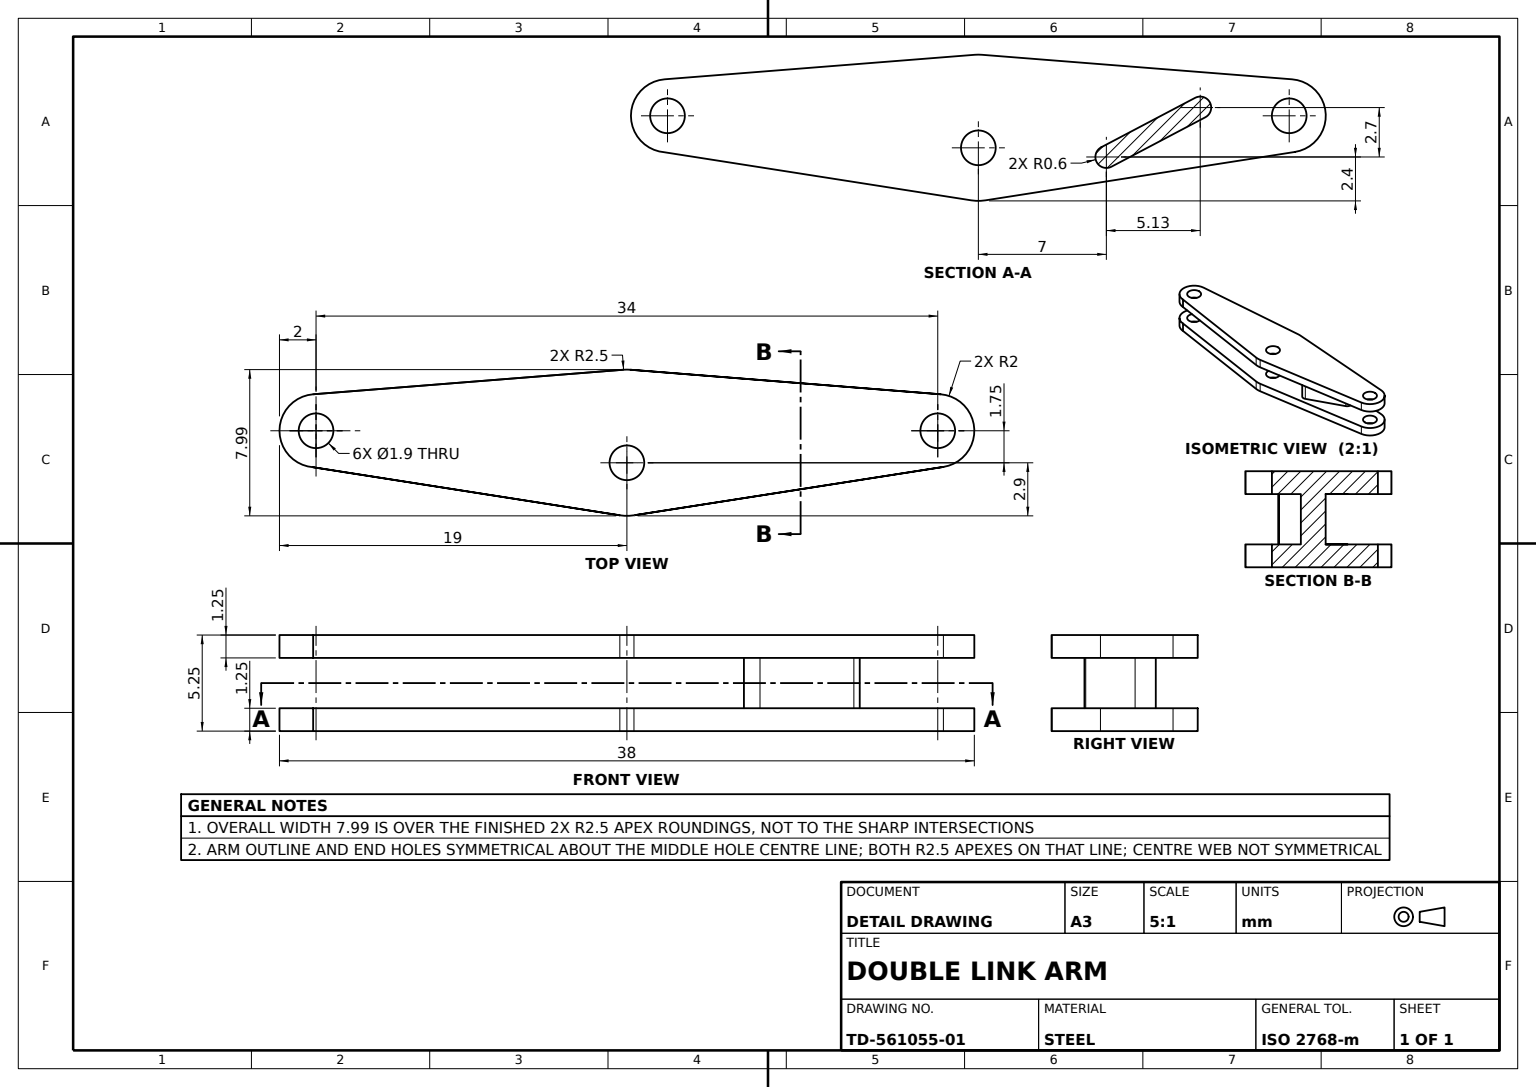
from build123d import *

# Parameters (mm, degrees)
ARM_PROFILE_SKETCH_R  = 0.95
ARM_BODY_DEPTH        = 2.625
FORK_SLOT_SKETCH_W    = 39.128483504
FORK_SLOT_SKETCH_H    = 2.75
FORK_SLOT_CUT_DEPTH   = 22.625
CENTRE_WEB_DEPTH      = 2.625
CENTRE_WEB_DEPTH_BACK = 1.375


with BuildPart() as part:
    # Arm Profile Sketch → Arm Body (new, symmetric)
    with BuildSketch(Plane(origin=(0, 0, 0), x_dir=(1, 0, 0), z_dir=(0, 1, 0))):
        with BuildLine():
            Line((-17.15759803, 1.993781046), (-0.196997537, 3.334428369))
            ThreePointArc((-0.196997537, 3.334428369), (0, 3.342202061), (0.196997537, 3.334428369))
            Line((0.196997537, 3.334428369), (17.15759803, 1.993781046))
            ThreePointArc((17.15759803, 1.993781046), (18.998552025, 0.076090769), (17.308740296, -1.976026171))
            Line((17.308740296, -1.976026171), (0.386342216, -4.620032749))
            ThreePointArc((0.386342216, -4.620032749), (0, -4.65), (-0.386332201, -4.619903915))
            Line((-0.386332201, -4.619903915), (-17.15759803, -1.993781046))
            ThreePointArc((-17.15759803, -1.993781046), (-19, 0), (-17.15759803, 1.993781046))
        make_face()
        with Locations(Location((-17, 0, 0), (0, 0, 90))):
            Circle(ARM_PROFILE_SKETCH_R, mode=Mode.SUBTRACT)
        with Locations(Location((17, 0, 0), (0, 0, 90))):
            Circle(ARM_PROFILE_SKETCH_R, mode=Mode.SUBTRACT)
        with Locations(Location((0, -1.75, 0), (0, 0, 90))):
            Circle(ARM_PROFILE_SKETCH_R, mode=Mode.SUBTRACT)
    extrude(amount=ARM_BODY_DEPTH, both=True)

    # Fork Slot Sketch → Fork Slot Cut (cut, symmetric)
    with BuildSketch(Plane.XY):
        Rectangle(FORK_SLOT_SKETCH_W, FORK_SLOT_SKETCH_H)
    extrude(amount=FORK_SLOT_CUT_DEPTH, both=True, mode=Mode.SUBTRACT)


with BuildPart() as fork_slot_cut_piece_1:
    # of the separate pieces the step leaves, piece 1, a body of its own (fork_slot_cut_pieces)
    add(part.part.solids().sort_by_distance((-0.386332201, -2.625, 4.619903915))[0])



with BuildPart() as fork_slot_cut_piece_2:
    # of the separate pieces the step leaves, piece 2, a body of its own (fork_slot_cut_pieces)
    add(part.part.solids().sort_by_distance((-0.386332201, 1.375, 4.619903915))[0])


with BuildPart() as fork_slot_cut_piece_1_1:
    add(fork_slot_cut_piece_1.part)

    add(fork_slot_cut_piece_2.part)  # Centre Web merges Fork Slot Cut piece 2
    # Centre Web Sketch → Centre Web (add, two sides: drawn at the far end of the back side and taken through both)
    with BuildSketch(Plane(origin=(0, 0, 0), x_dir=(1, 0, 0), z_dir=(0, 1, 0)).offset(-CENTRE_WEB_DEPTH_BACK)):
        with BuildLine():
            Line((6.720689655, -1.718976713), (11.853914762, 0.981023287))
            ThreePointArc((11.853914762, 0.981023287), (12.664248394, 0.729310345), (12.412535452, -0.081023287))
            Line((12.412535452, -0.081023287), (7.279310345, -2.781023287))
            ThreePointArc((7.279310345, -2.781023287), (6.468976713, -2.529310345), (6.720689655, -1.718976713))
        make_face()
    extrude(amount=CENTRE_WEB_DEPTH + CENTRE_WEB_DEPTH_BACK)


solid = fork_slot_cut_piece_1_1.part
